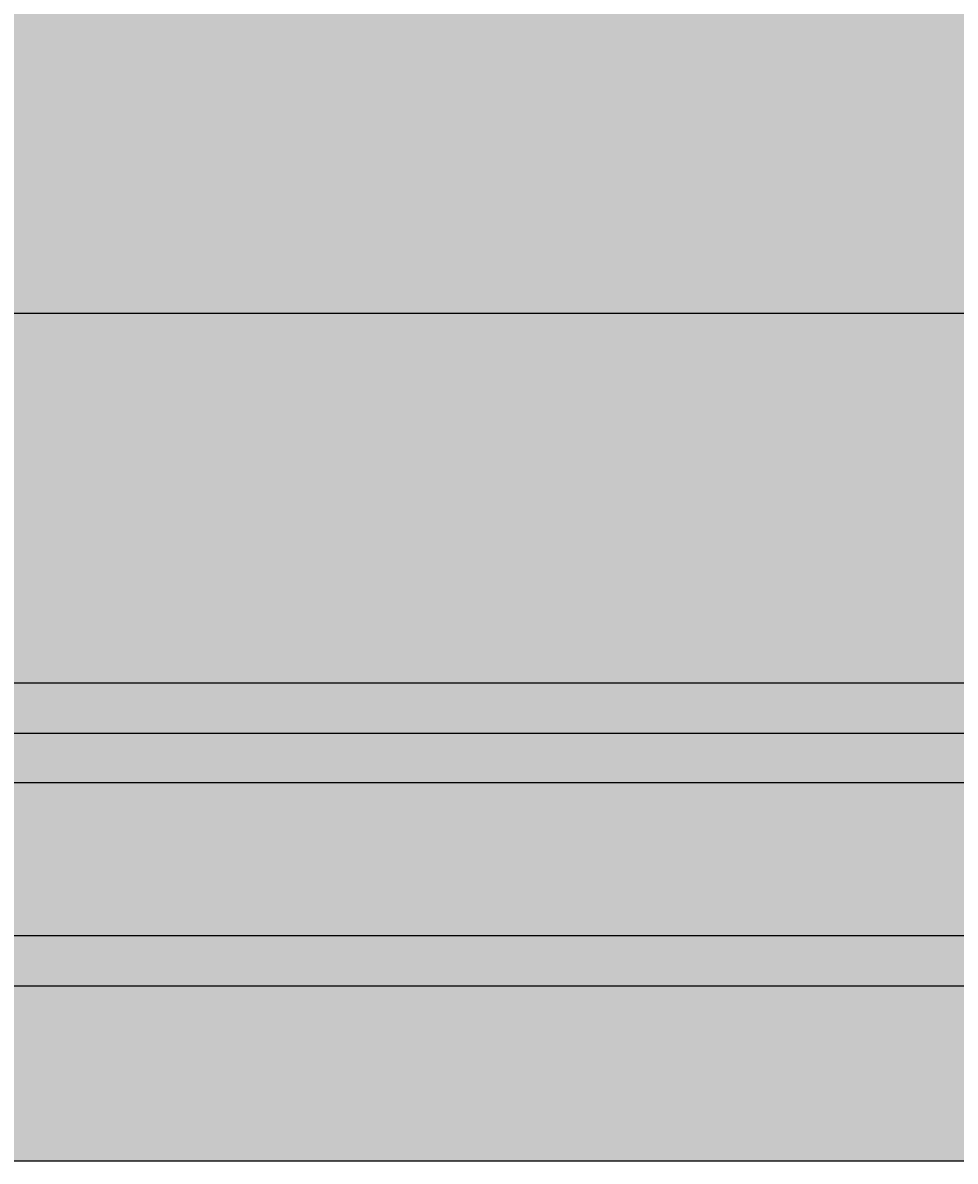
# Model space of a CAD drawing. Units: inches. Extents: x 35362 to 73946, y 43607 to 67532.
# Tile 59 of 134: x 46225 to 47763, y 46919 to 48798. Entities that reach past the tile are written whole.
import ezdxf

# ---------------------------------------------------------------- set-up
doc = ezdxf.new("R2010")
doc.units = ezdxf.units.IN
doc.header["$MEASUREMENT"] = 0
for name, color, linetype, lineweight in [('A-ANNO-DIMS', 2, 'Continuous', 18), ('E-SYMB', 1, 'Continuous', 25), ('E-SYMB-PATT', 1, 'Continuous', 13)]:
    doc.layers.add(name, color=color, linetype=linetype, lineweight=lineweight)
doc.styles.get("Standard").update_dxf_attribs({"font": 'arial.ttf'})
doc.dimstyles.get("Standard").update_dxf_attribs({"dimtxt": 0.18, "dimasz": 0.18, "dimexe": 0.18, "dimexo": 0.0625, "dimgap": 0.09, "dimtad": 0, "dimtih": 1, "dimtoh": 1, "dimdec": 4, "dimzin": 0, "dimdsep": 46, "dimtxsty": 'Standard', "dimcen": 0.09, "dimadec": 0, "dimazin": 0, "dimtfac": 1, "dimtdec": 4, "dimtofl": 0, "dimtmove": 0, "dimatfit": 3, "dimfxl": 1, "dimtolj": 1, "dimtzin": 0, "dimarcsym": 0})

# ---------------------------------------------------------------- blocks, each defined once
blk = doc.blocks.new('*D43')
at = {"layer": 'A-ANNO-DIMS', "color": 0, "lineweight": -2, "transparency": 16777216}
for p, q in [((62004.7, 47625.2), (35361.8, 47625.2)), ((35361.9, 47625), (35361.9, 47416.9)), ((35361.9, 47208.4), (35361.9, 47416.5)), ((62004.7, 47208.2), (35361.8, 47208.2))]:
    blk.add_line(p, q, dxfattribs=at)
at = {"layer": 'A-ANNO-DIMS', "color": 0, "transparency": 16777216}
for points in [[(35361.9, 47625), (35362, 47625), (35361.9, 47625.2)], [(35361.9, 47208.4), (35362, 47208.4), (35361.9, 47208.2)]]:
    blk.add_solid(points, dxfattribs=at)
at = {"layer": 'Defpoints', "color": 0, "transparency": 16777216}
for p in [(62004.7, 47625.2), (35361.9, 47208.2), (62004.7, 47208.2)]:
    blk.add_point(p, dxfattribs=at)
at = {"layer": 'A-ANNO-DIMS', "color": 0, "transparency": 16777216, "insert": (35361.9, 47416.7), "char_height": 0.18, "attachment_point": 5}
blk.add_mtext('\\A1;416.9', dxfattribs=at)
blk = doc.blocks.new('*D67')
at = {"layer": 'A-ANNO-DIMS', "color": 0, "lineweight": -2, "transparency": 16777216}
for p, q in [((56873.5, 53351.5), (35361.8, 53351.5)), ((35361.9, 53351.3), (35361.9, 49400.9)), ((35361.9, 45450.1), (35361.9, 49400.5)), ((53793.6, 45449.9), (35361.8, 45449.9))]:
    blk.add_line(p, q, dxfattribs=at)
at = {"layer": 'A-ANNO-DIMS', "color": 0, "transparency": 16777216}
for points in [[(35361.9, 53351.3), (35362, 53351.3), (35361.9, 53351.5)], [(35361.9, 45450.1), (35362, 45450.1), (35361.9, 45449.9)]]:
    blk.add_solid(points, dxfattribs=at)
at = {"layer": 'Defpoints', "color": 0, "transparency": 16777216}
for p in [(35361.9, 53351.5), (56873.6, 53351.5), (53793.6, 45449.9)]:
    blk.add_point(p, dxfattribs=at)
at = {"layer": 'A-ANNO-DIMS', "color": 0, "transparency": 16777216, "insert": (35361.9, 49400.7), "char_height": 0.18, "attachment_point": 5}
blk.add_mtext('\\A1;7901.6', dxfattribs=at)
blk = doc.blocks.new('*D87')
at = {"layer": 'A-ANNO-DIMS', "color": 0, "lineweight": -2, "transparency": 16777216}
for p, q in [((52362.5, 48318.3), (35361.8, 48318.3)), ((35361.9, 48318.1), (35361.9, 47931.4)), ((35361.9, 47544.3), (35361.9, 47931)), ((52362.5, 47544.1), (35361.8, 47544.1))]:
    blk.add_line(p, q, dxfattribs=at)
at = {"layer": 'A-ANNO-DIMS', "color": 0, "transparency": 16777216}
for points in [[(35361.9, 48318.1), (35362, 48318.1), (35361.9, 48318.3)], [(35361.9, 47544.3), (35362, 47544.3), (35361.9, 47544.1)]]:
    blk.add_solid(points, dxfattribs=at)
at = {"layer": 'Defpoints', "color": 0, "transparency": 16777216}
for p in [(35361.9, 48318.3), (52362.6, 48318.3), (52362.6, 47544.1)]:
    blk.add_point(p, dxfattribs=at)
at = {"layer": 'A-ANNO-DIMS', "color": 0, "transparency": 16777216, "insert": (35361.9, 47931.2), "char_height": 0.18, "attachment_point": 5}
blk.add_mtext('\\A1;774.1', dxfattribs=at)
blk = doc.blocks.new('*D89')
at = {"layer": 'A-ANNO-DIMS', "color": 0, "lineweight": -2, "transparency": 16777216}
for p, q in [((53707.7, 48897.7), (35361.8, 48897.7)), ((35361.9, 48897.6), (35361.9, 48303.2)), ((35361.9, 47708.4), (35361.9, 48302.8)), ((53707.7, 47708.2), (35361.8, 47708.2))]:
    blk.add_line(p, q, dxfattribs=at)
at = {"layer": 'A-ANNO-DIMS', "color": 0, "transparency": 16777216}
for points in [[(35361.9, 48897.6), (35362, 48897.6), (35361.9, 48897.7)], [(35361.9, 47708.4), (35362, 47708.4), (35361.9, 47708.2)]]:
    blk.add_solid(points, dxfattribs=at)
at = {"layer": 'Defpoints', "color": 0, "transparency": 16777216}
for p in [(53707.8, 48897.7), (35361.9, 47708.2), (53707.8, 47708.2)]:
    blk.add_point(p, dxfattribs=at)
at = {"layer": 'A-ANNO-DIMS', "color": 0, "transparency": 16777216, "insert": (35361.9, 48303), "char_height": 0.18, "attachment_point": 5}
blk.add_mtext('\\A1;1189.5', dxfattribs=at)
blk = doc.blocks.new('*D90')
at = {"layer": 'A-ANNO-DIMS', "color": 0, "lineweight": -2, "transparency": 16777216}
for p, q in [((53707.7, 47291.3), (35361.8, 47291.3)), ((35361.9, 47291.1), (35361.9, 46710.3)), ((35361.9, 46129.1), (35361.9, 46709.9)), ((53793.6, 46128.9), (35361.8, 46128.9))]:
    blk.add_line(p, q, dxfattribs=at)
at = {"layer": 'A-ANNO-DIMS', "color": 0, "transparency": 16777216}
for points in [[(35361.9, 47291.1), (35362, 47291.1), (35361.9, 47291.3)], [(35361.9, 46129.1), (35362, 46129.1), (35361.9, 46128.9)]]:
    blk.add_solid(points, dxfattribs=at)
at = {"layer": 'Defpoints', "color": 0, "transparency": 16777216}
for p in [(53707.8, 47291.3), (35361.9, 46128.9), (53793.6, 46128.9)]:
    blk.add_point(p, dxfattribs=at)
at = {"layer": 'A-ANNO-DIMS', "color": 0, "transparency": 16777216, "insert": (35361.9, 46710.1), "char_height": 0.18, "attachment_point": 5}
blk.add_mtext('\\A1;1162.4', dxfattribs=at)

msp = doc.modelspace()

# ---------------------------------------------------------------- hatches: boundary and pattern name
at = {"layer": 'E-SYMB-PATT'}
h = msp.add_hatch(color=256, dxfattribs=at)
h.dxf.hatch_style = 1
h.paths.add_polyline_path([(48163.038, 49689.843), (45390.147, 49689.843), (45390.147, 46919.381), (48163.038, 46919.381)])

# ---------------------------------------------------------------- linework, layer by layer
at = {"layer": 'E-SYMB'}
msp.add_lwpolyline([(45390.147, 49689.843), (48163.038, 49689.843), (48163.038, 46919.381), (45390.147, 46919.381)], close=True, dxfattribs=at)

# ---------------------------------------------------------------- dimensions: what is measured, and where the dimension line sits
at = {"layer": 'A-ANNO-DIMS'}
for base, p1, p2, picture, middle in [((35361.949, 53351.529), (53793.638, 45449.894), (56873.602, 53351.529), '*D67', (35361.949, 49400.712)), ((35361.949, 47708.216), (53707.781, 48897.738), (53707.781, 47708.216), '*D89', (35361.949, 48302.977)), ((35361.949, 48318.269), (52362.557, 47544.134), (52362.557, 48318.269), '*D87', (35361.949, 47931.201)), ((35361.949, 47208.25), (62004.728, 47625.181), (62004.728, 47208.25), '*D43', (35361.949, 47416.715)), ((35361.949, 46128.878), (53707.781, 47291.285), (53793.638, 46128.878), '*D90', (35361.949, 46710.081))]:
    dim = msp.add_linear_dim(base=base, p1=p1, p2=p2, angle=90, dimstyle='Standard', override={"dimdec": 1, "dimlfac": 1, "dimrnd": 0, "dimzin": 0, "dimdsep": 46, "dimlunit": 2}, dxfattribs=at)
    dim.commit()
    dim.dimension.update_dxf_attribs({"geometry": picture, "text_midpoint": middle})

doc.saveas('drawing.dxf')
